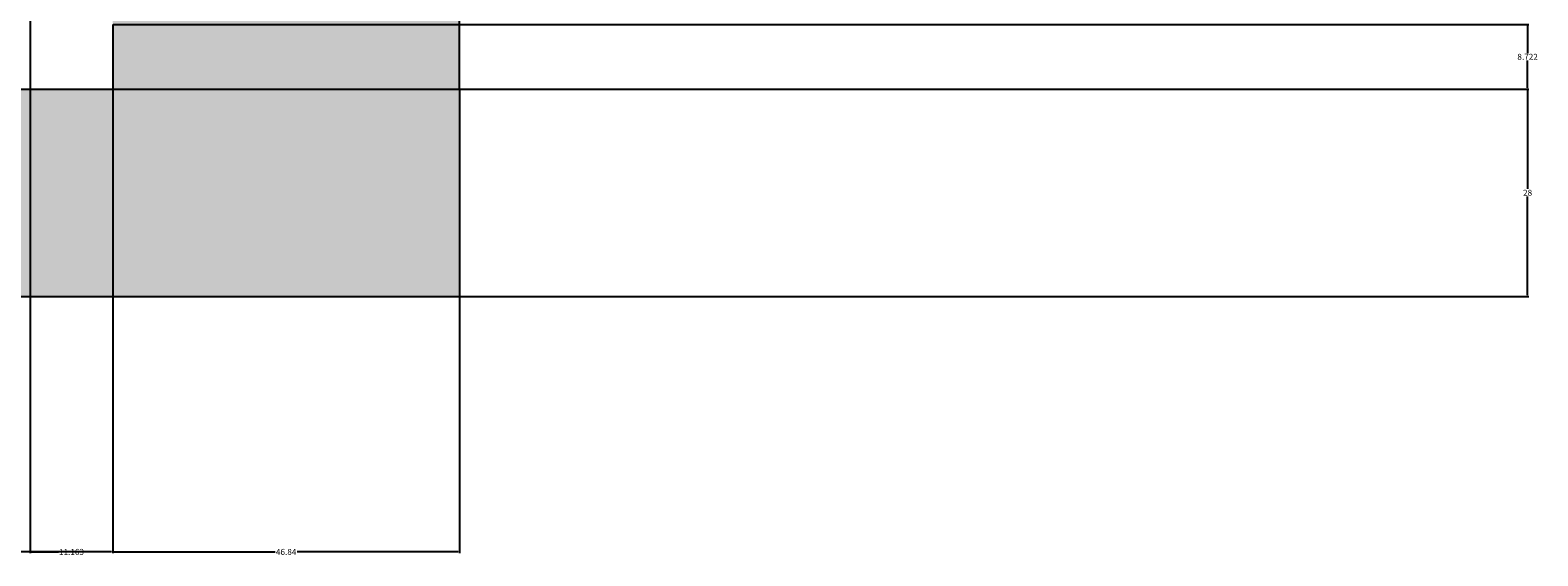
# Model space of a CAD drawing. Units: inches. Extents: x 36 to 594, y 79 to 831.
# Tile 11 of 30: x 390 to 594, y 79 to 150. Entities that reach past the tile are written whole.
import ezdxf

# ---------------------------------------------------------------- set-up
doc = ezdxf.new("R2010")
doc.units = ezdxf.units.IN
doc.header["$MEASUREMENT"] = 0
for name, color, linetype, lineweight in [('A-ANNO-DIMS', 2, 'Continuous', 18), ('A-ELEV', 7, 'Continuous', 25), ('A-ELEV-PATT', 8, 'Continuous', 13)]:
    doc.layers.add(name, color=color, linetype=linetype, lineweight=lineweight)
doc.styles.get("Standard").update_dxf_attribs({"font": 'arial.ttf'})
doc.dimstyles.get("Standard").update_dxf_attribs({"dimtxt": 0.8125, "dimasz": 0.18, "dimexe": 0.18, "dimexo": 0.0625, "dimgap": 0.09, "dimtad": 0, "dimtih": 1, "dimtoh": 1, "dimdec": 4, "dimzin": 0, "dimdsep": 46, "dimlunit": 4, "dimtxsty": 'Standard', "dimcen": 0.09, "dimadec": 0, "dimazin": 0, "dimtfac": 1, "dimtdec": 4, "dimtofl": 0, "dimtmove": 0, "dimatfit": 3, "dimfxl": 1, "dimtolj": 1, "dimtzin": 0, "dimarcsym": 0})

# ---------------------------------------------------------------- blocks, each defined once
blk = doc.blocks.new('*D10')
at = {"layer": 'A-ANNO-DIMS', "color": 0, "lineweight": -2, "transparency": 16777216}
for p, q in [((254.03, 142.15), (254.03, 79.53)), ((401.55, 142.15), (401.55, 79.53)), ((254.21, 79.71), (326.06, 79.71)), ((401.37, 79.71), (329.52, 79.71))]:
    blk.add_line(p, q, dxfattribs=at)
at = {"layer": 'A-ANNO-DIMS', "color": 0, "transparency": 16777216}
for points in [[(254.21, 79.74), (254.21, 79.68), (254.03, 79.71)], [(401.37, 79.74), (401.37, 79.68), (401.55, 79.71)]]:
    blk.add_solid(points, dxfattribs=at)
at = {"layer": 'Defpoints', "color": 0, "transparency": 16777216}
for p in [(254.03, 142.21), (401.55, 142.21), (401.55, 79.71)]:
    blk.add_point(p, dxfattribs=at)
at = {"layer": 'A-ANNO-DIMS', "color": 0, "transparency": 16777216, "insert": (327.79, 79.71), "char_height": 0.812, "attachment_point": 5}
blk.add_mtext('\\A1;147.52', dxfattribs=at)
blk = doc.blocks.new('*D11')
at = {"layer": 'A-ANNO-DIMS', "color": 0, "lineweight": -2, "transparency": 16777216}
for p, q in [((401.55, 142.15), (401.55, 79.53)), ((448.39, 114.15), (448.39, 79.53)), ((401.73, 79.71), (423.49, 79.71)), ((448.21, 79.71), (426.45, 79.71))]:
    blk.add_line(p, q, dxfattribs=at)
at = {"layer": 'A-ANNO-DIMS', "color": 0, "transparency": 16777216}
for points in [[(401.73, 79.74), (401.73, 79.68), (401.55, 79.71)], [(448.21, 79.74), (448.21, 79.68), (448.39, 79.71)]]:
    blk.add_solid(points, dxfattribs=at)
at = {"layer": 'Defpoints', "color": 0, "transparency": 16777216}
for p in [(401.55, 142.21), (448.39, 114.21), (448.39, 79.71)]:
    blk.add_point(p, dxfattribs=at)
at = {"layer": 'A-ANNO-DIMS', "color": 0, "transparency": 16777216, "insert": (424.97, 79.71), "char_height": 0.812, "attachment_point": 5}
blk.add_mtext('\\A1;46.84', dxfattribs=at)
blk = doc.blocks.new('*D29')
at = {"layer": 'A-ANNO-DIMS', "color": 0, "lineweight": -2, "transparency": 16777216}
for p, q in [((401.61, 142.21), (592.85, 142.21)), ((592.67, 142.03), (592.67, 128.72)), ((592.67, 114.39), (592.67, 127.71)), ((448.45, 114.21), (592.85, 114.21))]:
    blk.add_line(p, q, dxfattribs=at)
at = {"layer": 'A-ANNO-DIMS', "color": 0, "transparency": 16777216}
for points in [[(592.64, 142.03), (592.7, 142.03), (592.67, 142.21)], [(592.64, 114.39), (592.7, 114.39), (592.67, 114.21)]]:
    blk.add_solid(points, dxfattribs=at)
at = {"layer": 'Defpoints', "color": 0, "transparency": 16777216}
for p in [(401.55, 142.21), (592.67, 142.21), (448.39, 114.21)]:
    blk.add_point(p, dxfattribs=at)
at = {"layer": 'A-ANNO-DIMS', "color": 0, "transparency": 16777216, "insert": (592.67, 128.21), "char_height": 0.812, "attachment_point": 5}
blk.add_mtext('\\A1;28', dxfattribs=at)
blk = doc.blocks.new('*D30')
at = {"layer": 'A-ANNO-DIMS', "color": 0, "lineweight": -2, "transparency": 16777216}
for p, q in [((401.61, 150.93), (592.85, 150.93)), ((592.67, 150.75), (592.67, 147.08)), ((592.67, 142.39), (592.67, 146.07)), ((401.61, 142.21), (592.85, 142.21))]:
    blk.add_line(p, q, dxfattribs=at)
at = {"layer": 'A-ANNO-DIMS', "color": 0, "transparency": 16777216}
for points in [[(592.64, 150.75), (592.7, 150.75), (592.67, 150.93)], [(592.64, 142.39), (592.7, 142.39), (592.67, 142.21)]]:
    blk.add_solid(points, dxfattribs=at)
at = {"layer": 'Defpoints', "color": 0, "transparency": 16777216}
for p in [(401.55, 150.93), (592.67, 150.93), (401.55, 142.21)]:
    blk.add_point(p, dxfattribs=at)
at = {"layer": 'A-ANNO-DIMS', "color": 0, "transparency": 16777216, "insert": (592.67, 146.57), "char_height": 0.812, "attachment_point": 5}
blk.add_mtext('\\A1;8.722', dxfattribs=at)
blk = doc.blocks.new('*D82')
at = {"layer": 'A-ANNO-DIMS', "color": 0, "lineweight": -2, "transparency": 16777216}
for p, q in [((335.35, 162.93), (335.35, 79.53)), ((390.39, 162.93), (390.39, 79.53)), ((335.53, 79.71), (361.41, 79.71)), ((390.21, 79.71), (364.33, 79.71))]:
    blk.add_line(p, q, dxfattribs=at)
at = {"layer": 'A-ANNO-DIMS', "color": 0, "transparency": 16777216}
for points in [[(335.53, 79.74), (335.53, 79.68), (335.35, 79.71)], [(390.21, 79.74), (390.21, 79.68), (390.39, 79.71)]]:
    blk.add_solid(points, dxfattribs=at)
at = {"layer": 'Defpoints', "color": 0, "transparency": 16777216}
for p in [(335.35, 162.99), (390.39, 162.99), (390.39, 79.71)]:
    blk.add_point(p, dxfattribs=at)
at = {"layer": 'A-ANNO-DIMS', "color": 0, "transparency": 16777216, "insert": (362.87, 79.71), "char_height": 0.812, "attachment_point": 5}
blk.add_mtext('\\A1;55.04', dxfattribs=at)
blk = doc.blocks.new('*D83')
at = {"layer": 'A-ANNO-DIMS', "color": 0, "lineweight": -2, "transparency": 16777216}
for p, q in [((390.39, 162.93), (390.39, 79.53)), ((401.55, 150.87), (401.55, 79.53)), ((390.57, 79.71), (394.23, 79.71)), ((401.37, 79.71), (397.71, 79.71))]:
    blk.add_line(p, q, dxfattribs=at)
at = {"layer": 'A-ANNO-DIMS', "color": 0, "transparency": 16777216}
for points in [[(390.57, 79.74), (390.57, 79.68), (390.39, 79.71)], [(401.37, 79.74), (401.37, 79.68), (401.55, 79.71)]]:
    blk.add_solid(points, dxfattribs=at)
at = {"layer": 'Defpoints', "color": 0, "transparency": 16777216}
for p in [(390.39, 162.99), (401.55, 150.93), (401.55, 79.71)]:
    blk.add_point(p, dxfattribs=at)
at = {"layer": 'A-ANNO-DIMS', "color": 0, "transparency": 16777216, "insert": (395.97, 79.71), "char_height": 0.812, "attachment_point": 5}
blk.add_mtext('\\A1;11.163', dxfattribs=at)

msp = doc.modelspace()

# ---------------------------------------------------------------- hatches: boundary and pattern name
at = {"layer": 'A-ELEV-PATT'}
h = msp.add_hatch(color=256, dxfattribs=at)
h.dxf.hatch_style = 1
h.paths.add_polyline_path([(398.0873, 796.0465), (269.3592, 796.0465), (269.3592, 770.1455), (397.8159, 770.1455)])
h.paths.add_polyline_path([(397.7518, 764.0341), (269.3592, 764.0341), (269.3592, 630.0394), (341.8367, 630.0394), (341.8367, 720.595), (335.0881, 728.3699), (329.982, 735.3373), (345.3661, 727.7743), (397.1052, 702.3389)])
h.paths.add_polyline_path([(341.8367, 594.2124), (201.4189, 594.2124), (201.4189, 475.4136), (232.8216, 475.4136), (232.8216, 524.6037), (341.8367, 524.6037)])
h.paths.add_polyline_path([(177.525, 594.2124), (118.7598, 594.2124), (118.7598, 450.2124), (177.525, 450.2124)])
h.paths.add_polyline_path([(424.4958, 594.2124), (365.7306, 594.2124), (365.7306, 450.2124), (424.4958, 450.2124)])
h.paths.add_polyline_path([(241.3553, 404.2737), (355.8569, 404.2737), (355.8569, 355.0836), (424.5492, 355.0836), (424.5492, 425.7333), (118.7598, 426.2844), (118.7598, 355.0836), (241.3553, 355.0836)])
h.paths.add_polyline_path([(448.3898, 306.2124), (217.0273, 306.2124), (217.0273, 142.2124), (254.0293, 142.2124), (254.0293, 150.9347), (254.0293, 286.1802), (401.5491, 286.1802), (401.5491, 150.9347), (401.5491, 142.2124), (448.3898, 142.2124)])
h.paths.add_polyline_path([(448.3898, 142.2124), (401.5491, 142.2124), (217.0273, 142.2124), (217.0273, 114.2124), (448.3898, 114.2124)])
h.paths.add_polyline_path([(217.0273, 306.2124), (174.7353, 306.2124), (94.8658, 306.2124), (94.8658, 162.2124), (103.3368, 162.2124), (103.3368, 264.6224), (103.3368, 286.1802), (217.0273, 286.1802)])

# ---------------------------------------------------------------- linework, layer by layer
at = {"layer": 'A-ELEV'}
for p, q in [((448.3898, 142.2124), (448.3898, 367.5118)), ((401.5491, 150.9347), (401.5491, 142.2124)), ((174.7353, 142.2124), (448.3898, 142.2124)), ((448.3898, 142.2124), (448.3898, 114.2124)), ((84.3711, 114.2124), (558.1689, 114.2124))]:
    msp.add_line(p, q, dxfattribs=at)

# ---------------------------------------------------------------- dimensions: what is measured, and where the dimension line sits
at = {"layer": 'A-ANNO-DIMS'}
for base, p1, p2, override, picture, middle in [((390.386, 79.7124), (335.3496, 162.9881), (390.386, 162.9881), {"dimdec": 2, "dimlfac": 1, "dimrnd": 0, "dimzin": 0, "dimdsep": 46, "dimlunit": 2}, '*D82', (362.8678, 79.7124)), ((401.5491, 79.7124), (390.386, 162.9881), (401.5491, 150.9347), {"dimdec": 3, "dimlfac": 1, "dimrnd": 0, "dimzin": 0, "dimdsep": 46, "dimlunit": 2}, '*D83', (395.9676, 79.7124)), ((401.5491, 79.7124), (254.0293, 142.2124), (401.5491, 142.2124), {"dimdec": 2, "dimlfac": 1, "dimrnd": 0, "dimzin": 0, "dimdsep": 46, "dimlunit": 2}, '*D10', (327.7892, 79.7124)), ((448.3898, 79.7124), (401.5491, 142.2124), (448.3898, 114.2124), {"dimdec": 2, "dimlfac": 1, "dimrnd": 0, "dimzin": 0, "dimdsep": 46, "dimlunit": 2}, '*D11', (424.9694, 79.7124))]:
    dim = msp.add_linear_dim(base=base, p1=p1, p2=p2, dimstyle='Standard', override=override, dxfattribs=at)
    dim.commit()
    dim.dimension.update_dxf_attribs({"geometry": picture, "text_midpoint": middle})
for base, p1, p2, override, picture, middle in [((592.6689, 150.9347), (401.5491, 142.2124), (401.5491, 150.9347), {"dimdec": 3, "dimlfac": 1, "dimrnd": 0, "dimzin": 0, "dimdsep": 46, "dimlunit": 2}, '*D30', (592.6689, 146.5735)), ((592.6689, 142.2124), (448.3898, 114.2124), (401.5491, 142.2124), {"dimdec": 0, "dimlfac": 1, "dimrnd": 0, "dimzin": 0, "dimdsep": 46, "dimlunit": 2}, '*D29', (592.6689, 128.2124))]:
    dim = msp.add_linear_dim(base=base, p1=p1, p2=p2, angle=90, dimstyle='Standard', override=override, dxfattribs=at)
    dim.commit()
    dim.dimension.update_dxf_attribs({"geometry": picture, "text_midpoint": middle})

doc.saveas('drawing.dxf')
